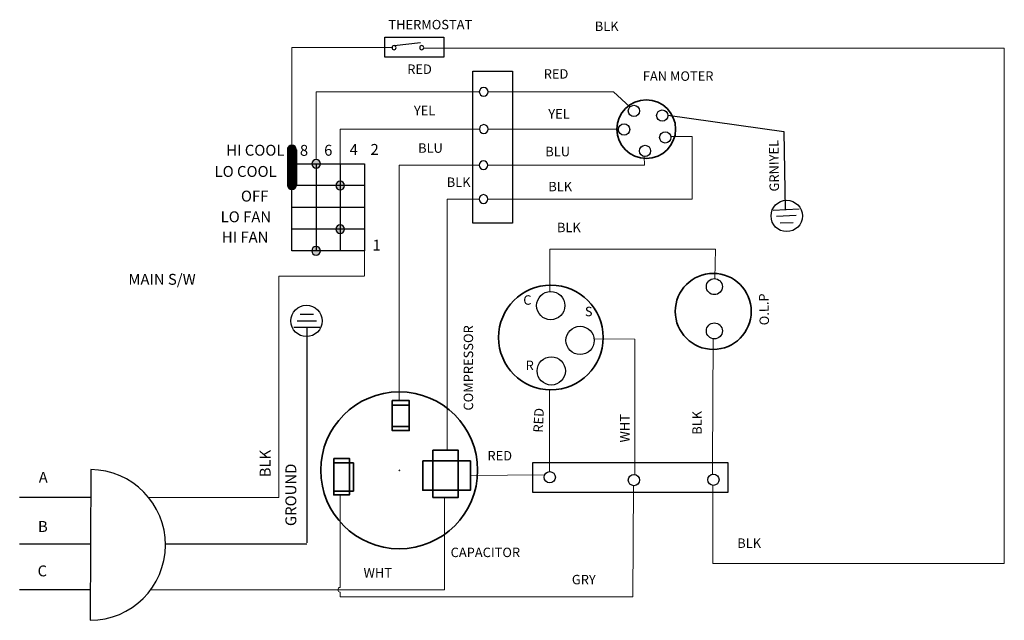
# Model space of a CAD drawing. Units: inches. Extents: x 2585 to 4283, y 904 to 1939.
import ezdxf

# ---------------------------------------------------------------- set-up
doc = ezdxf.new("R2010")
doc.units = ezdxf.units.IN
doc.header["$MEASUREMENT"] = 0
for name, color, linetype, lineweight in [('E-ANNO-TEXT', 7, 'Continuous', 25), ('E-POWR-EQPM', 7, 'Continuous', 35), ('E-POWR-GRND', 3, 'Continuous', 25), ('E-POWR-PATT', 7, 'Continuous', 13), ('E-POWR-SWCH', 7, 'Continuous', 30), ('E-POWR-TERM', 7, 'Continuous', 25), ('E-POWR-WIRE', 7, 'Continuous', 18), ('E-WIRE-TEXT', 7, 'Continuous', 18)]:
    doc.layers.add(name, color=color, linetype=linetype, lineweight=lineweight)
doc.styles.get("Standard").update_dxf_attribs({"font": 'arial.ttf'})

# ---------------------------------------------------------------- blocks, each defined once
blk = doc.blocks.new('Ground')
for p, q in [((-0.1, 0), (0.1, 0)), ((0.075, -0.05), (-0.075, -0.05)), ((-0.05, -0.1), (0.05, -0.1))]:
    blk.add_line(p, q)
blk = doc.blocks.new('GROUND-CIRCLED')
blk.add_circle((27, 27), 27)
at = {"xscale": 225.3922525633989, "yscale": 225.3922525633989, "zscale": 225.3922525633989, "rotation": 180}
blk.add_blockref('Ground', (27.6, 15.9), dxfattribs=at)
blk = doc.blocks.new('TERMINAL-STRIP-CONTACT')
blk.add_lwpolyline([(0, 7.5, 1), (15, 7.5, 1)], format="xyb", close=True)
blk = doc.blocks.new('TERMINAL-OPEN')
blk.add_circle((9.8, 9.8), 9.75)
blk = doc.blocks.new('SELECTOR-CONTACT')
blk.add_lwpolyline([(0, 7.5, 1), (15, 7.5, 1)], format="xyb", close=True)
blk = doc.blocks.new('COMPRESSOR-TERMINAL')
blk.add_circle((24.4, 24.4), 24.4)
blk = doc.blocks.new('OVERLOAD-TERMINAL')
blk.add_circle((13.8, 13.8), 13.8)

msp = doc.modelspace()

# ---------------------------------------------------------------- hatches: boundary and pattern name
at = {"layer": 'E-POWR-PATT'}
h = msp.add_hatch(dxfattribs=at)
h.set_pattern_fill('ANSI31', color=256)
h.set_pattern_definition([(45, (2034.52184, 1087.94078), (-0.088388348, 0.088388348), [])])
h.paths.add_polyline_path([(3054.4, 1690.8), (3054.4, 1722.8, 0.417432), (3046.6, 1715.1), (3046.6, 1654.3, 0.417432), (3054.4, 1646.6)])
h.paths.add_polyline_path([(3062.1, 1690.8), (3054.4, 1690.8), (3054.4, 1646.6, 0.411002), (3062.1, 1654.3)])
h.paths.add_polyline_path([(3062.1, 1715.1, 0.411002), (3054.4, 1722.8), (3054.4, 1690.8), (3062.1, 1690.8)])
h = msp.add_hatch(color=256, dxfattribs=at)
h.dxf.hatch_style = 1
h.paths.add_polyline_path([(3088.7, 1690.8), (3103.7, 1690.8, 1)])
h.paths.add_polyline_path([(3103.7, 1690.8), (3096.2, 1690.8), (3096.2, 1683.3, 0.414214)])
h.paths.add_polyline_path([(3096.2, 1690.8), (3088.7, 1690.8, 0.414214), (3096.2, 1683.3)])
h.paths.add_polyline_path([(3137.9, 1585.7, 0.414214), (3130.4, 1578.2), (3137.9, 1578.2)])
h.paths.add_polyline_path([(3137.9, 1585.7), (3137.9, 1578.2), (3145.4, 1578.2, 0.414214)])
h.paths.add_polyline_path([(3145.4, 1578.2), (3137.9, 1578.2), (3137.9, 1570.7, 0.414214)])
h.paths.add_polyline_path([(3137.9, 1578.2), (3130.4, 1578.2, 0.414214), (3137.9, 1570.7)])
h.paths.add_polyline_path([(3145.4, 1653.2), (3137.9, 1653.2), (3137.9, 1645.7, 0.414214)])
h.paths.add_polyline_path([(3137.9, 1653.2), (3130.4, 1653.2, 0.414214), (3137.9, 1645.7)])
h.paths.add_polyline_path([(3137.9, 1660.7, 0.414214), (3130.4, 1653.2), (3137.9, 1653.2)])
h.paths.add_polyline_path([(3137.9, 1660.7), (3137.9, 1653.2), (3145.4, 1653.2, 0.414214)])
h.paths.add_polyline_path([(3103.7, 1540.7), (3088.7, 1540.7, 1)])
h.paths.add_polyline_path([(3096.2, 1548.2), (3096.2, 1540.7), (3103.7, 1540.7, 0.414214)])
h.paths.add_polyline_path([(3096.2, 1548.2, 0.414214), (3088.7, 1540.7), (3096.2, 1540.7)])

# ---------------------------------------------------------------- linework, layer by layer
at = {"layer": 'E-POWR-EQPM'}
for p, q in [((3227.4, 1274.9), (3257.3, 1274.9)), ((3227.5, 1237.8), (3256.5, 1237.8)), ((3126.5, 1175), (3160.8, 1175)), ((3160.8, 1175), (3160.8, 1126.1)), ((3160.8, 1126.1), (3126.3, 1126.1))]:
    msp.add_line(p, q, dxfattribs=at)
for points in [[(3227.4, 1282.5), (3256.9, 1282.5), (3256.9, 1230.7), (3227.4, 1230.7)], [(3297.6, 1196.8), (3341.4, 1196.8), (3341.4, 1115.5), (3297.6, 1115.5)], [(3126.5, 1182.8), (3153.5, 1182.8), (3153.5, 1120), (3126.5, 1120)], [(3280.1, 1178.5), (3362.4, 1178.5), (3362.4, 1127.8), (3280.1, 1127.8)]]:
    msp.add_lwpolyline(points, close=True, dxfattribs=at)
for centre, radius in [((3665.7, 1750.4), 50.6), ((3781.2, 1436.3), 65.5), ((3501.1, 1391.3), 90.2), ((3239.5, 1162.3), 135.3), ((3239.8, 1162.3), 0.287)]:
    msp.add_circle(centre, radius, dxfattribs=at)
at = {"layer": 'E-POWR-GRND'}
for p, q in [((3702.9, 1774.4), (3902.7, 1746.4)), ((3902.7, 1746.5), (3905.3, 1611.8)), ((3080.4, 1408.5), (3080.4, 1340.3)), ((3080.4, 1344.6), (3080.4, 1037.1)), ((3080.4, 1034.9), (2836.3, 1034.9))]:
    msp.add_line(p, q, dxfattribs=at)
at = {"layer": 'E-POWR-SWCH'}
for p, q in [((3230.6, 1894.6), (3276.1, 1900.1)), ((3046.6, 1715.1), (3046.6, 1654.3)), ((3062.1, 1715.1), (3062.1, 1654.3)), ((3054.4, 1690.8), (3179.5, 1690.8)), ((3054.4, 1540.7), (3054.4, 1690.8)), ((3096.2, 1690.8), (3096.2, 1540.7)), ((3137.9, 1690.8), (3137.9, 1540.7)), ((3179.5, 1690.8), (3179.5, 1540.7)), ((3179.5, 1653.2), (3054.4, 1653.2)), ((3179.5, 1615.7), (3054.4, 1615.7)), ((3179.5, 1578.2), (3054.4, 1578.2)), ((3179.5, 1540.7), (3054.4, 1540.7))]:
    msp.add_line(p, q, dxfattribs=at)
msp.add_lwpolyline([(3214.9, 1908.9), (3316.3, 1908.9), (3316.3, 1874.6), (3214.9, 1874.6)], close=True, dxfattribs=at)
for points in [[(3227.1, 1891.1, 1), (3234.1, 1891.1, 1)], [(3274.9, 1891.1, 1), (3281.9, 1891.1, 1)]]:
    msp.add_lwpolyline(points, format="xyb", close=True, dxfattribs=at)
for centre, start, end in [((3054.3, 1715.1), 0, 180), ((3054.3, 1654.3), 180, 0)]:
    msp.add_arc(centre, 7.74, start, end, dxfattribs=at)
at = {"layer": 'E-POWR-TERM'}
for p, q in [((2707.6, 1163.5), (2706.4, 903.7)), ((2707.4, 1115.5), (2584.8, 1115.5)), ((2707, 1034.9), (2584.8, 1034.9)), ((2706.6, 956.3), (2584.8, 956.3))]:
    msp.add_line(p, q, dxfattribs=at)
for points in [[(3366.6, 1850.5), (3434.8, 1850.5), (3434.8, 1588.3), (3366.6, 1588.3)], [(3470, 1175.7), (3806.4, 1175.7), (3806.4, 1123.8), (3470, 1123.8)]]:
    msp.add_lwpolyline(points, close=True, dxfattribs=at)
msp.add_arc((2706.4, 1033.6), 129.9, 270, 89.4511, dxfattribs=at)
at = {"layer": 'E-POWR-WIRE'}
for p, q in [((3227.1, 1891.1), (3054.4, 1891.1)), ((3054.4, 1891.1), (3054.4, 1690.8)), ((3281.8, 1890.2), (4283.3, 1890.2)), ((4283.3, 1001.7), (4283.3, 1890.2)), ((3096.2, 1698.3), (3096.2, 1815)), ((3096.2, 1815), (3377.9, 1815)), ((3392.7, 1815), (3609.2, 1815)), ((3609.2, 1815), (3637.6, 1788.9)), ((3609.2, 1815), (3609.2, 1815)), ((3137.9, 1690.8), (3137.9, 1750.7)), ((3137.9, 1750.7), (3378.6, 1750.7)), ((3393.1, 1750.8), (3617.5, 1750.8)), ((3745, 1737.8), (3708, 1737.9)), ((3745, 1630.1), (3745, 1737.8)), ((3662.4, 1688.4), (3662.3, 1703.2)), ((3377.7, 1688.5), (3239.5, 1688.5)), ((3239.5, 1688.5), (3239.5, 1282.5)), ((3392.7, 1688.5), (3608.3, 1688.5)), ((3608.3, 1688.5), (3645.1, 1688.4)), ((3643.5, 1688.4), (3662.4, 1688.4)), ((3377.7, 1630.1), (3322.2, 1630.1)), ((3322.2, 1630.1), (3322.2, 1196.8)), ((3392.7, 1630.1), (3606.6, 1630.1)), ((3606.6, 1630.1), (3745, 1630.1)), ((3179.5, 1540.7), (3179.5, 1497.7)), ((3499.2, 1543.4), (3499.1, 1470.6)), ((3779.9, 1543.4), (3499.2, 1543.4)), ((3779.3, 1543.4), (3784.9, 1543.4)), ((3784.9, 1543.4), (3783.9, 1492.8)), ((3179.5, 1497.2), (3032.1, 1497.2)), ((3032.1, 1497.2), (3032.1, 1115.5)), ((3646, 1388.4), (3575.8, 1389.1)), ((3646, 1155), (3646, 1388.4)), ((3779.9, 1175.5), (3780.8, 1389)), ((3498.8, 1301.1), (3498.8, 1159.9)), ((3779.9, 1155.6), (3779.9, 1175.7)), ((3362.4, 1153.6), (3490.2, 1154.3)), ((3642.4, 944.1), (3643.8, 1135.7)), ((3780.7, 1136.3), (3780.7, 1001.7)), ((3032.1, 1115.5), (2807.2, 1115.5)), ((3137.6, 1120), (3137.6, 960.3)), ((3317.7, 1115.5), (3317.7, 956.3)), ((3780.7, 1001.7), (4283.3, 1001.7)), ((3317.7, 956.3), (2810.8, 956.3)), ((3137.6, 952.2), (3137.6, 944.1)), ((3137.6, 944.1), (3642.4, 944.1))]:
    msp.add_line(p, q, dxfattribs=at)
msp.add_arc((3137.7, 956.3), 4.04, 91.3808, 268.6192, dxfattribs=at)

# ---------------------------------------------------------------- block references
at = {"layer": 'E-POWR-GRND', "rotation": 182.5618974607787}
msp.add_blockref('GROUND-CIRCLED', (3933.7, 1629), dxfattribs=at)
at = {"layer": 'E-POWR-GRND'}
msp.add_blockref('GROUND-CIRCLED', (3052.5, 1392.8), dxfattribs=at)
at = {"layer": 'E-POWR-SWCH'}
msp.add_blockref('SELECTOR-CONTACT', (3088.7, 1683.3), dxfattribs=at)
at = {"layer": 'E-POWR-SWCH', "rotation": 180}
for p in [(3145.1, 1660.7), (3145.1, 1585.7), (3103.5, 1548.2)]:
    msp.add_blockref('SELECTOR-CONTACT', p, dxfattribs=at)
at = {"layer": 'E-POWR-TERM'}
for name, p in [('TERMINAL-STRIP-CONTACT', (3377.7, 1807.5)), ('TERMINAL-OPEN', (3634.6, 1772.1)), ('TERMINAL-OPEN', (3683.4, 1764.1)), ('TERMINAL-OPEN', (3617.5, 1740.1)), ('TERMINAL-OPEN', (3688.6, 1726.5)), ('TERMINAL-OPEN', (3653.7, 1703.2)), ('OVERLOAD-TERMINAL', (3769.3, 1465.2)), ('COMPRESSOR-TERMINAL', (3476.5, 1421.9)), ('COMPRESSOR-TERMINAL', (3527.2, 1361.8)), ('OVERLOAD-TERMINAL', (3769.3, 1388.8)), ('COMPRESSOR-TERMINAL', (3477.4, 1309.3)), ('TERMINAL-OPEN', (3489.3, 1140.4)), ('TERMINAL-OPEN', (3634.6, 1135.6)), ('TERMINAL-OPEN', (3771.7, 1136.2))]:
    msp.add_blockref(name, p, dxfattribs=at)
at = {"layer": 'E-POWR-TERM', "rotation": 180}
for p in [(3392.8, 1758.3), (3392.5, 1696), (3392.5, 1637.6)]:
    msp.add_blockref('TERMINAL-STRIP-CONTACT', p, dxfattribs=at)

# ---------------------------------------------------------------- texts
at = {"layer": 'E-ANNO-TEXT'}
for s, height, p in [('THERMOSTAT', 16.29, (3220.9, 1922.7)), ('FAN MOTER', 16.29, (3659.7, 1833.9)), ('HI COOL', 18.81, (2941.2, 1704.8)), ('8', 18.8, (3068.2, 1704.6)), ('6', 18.8, (3110, 1704.8)), ('4', 18.8, (3154, 1705.9)), ('2', 18.8, (3190, 1706.2)), ('LO COOL', 18.81, (2921, 1668.2)), ('OFF', 18.81, (2966.5, 1625.7)), ('LO FAN', 18.81, (2931.5, 1590)), ('HI FAN', 18.81, (2933.6, 1555)), ('1', 18.8, (3193.4, 1541.1)), ('MAIN S/W', 18.81, (2772.3, 1482.2)), ('C', 16.3, (3453.5, 1447.8)), ('S', 16.3, (3559.7, 1428)), ('R', 16.3, (3457.6, 1335)), ('A', 18.8, (2617.7, 1140.7)), ('B', 18.8, (2616.4, 1056)), ('CAPACITOR', 16.29, (3328.2, 1012.6)), ('C', 18.8, (2615.7, 979.4))]:
    msp.add_text(s, height=height, dxfattribs=at).set_placement(p)
for s, rotation, p in [('O.L.P', 91.2279, (3877.5, 1412.5)), ('COMPRESSOR', 90, (3367, 1265.3))]:
    msp.add_text(s, height=16.29, rotation=rotation, dxfattribs=at).set_placement(p)
at = {"layer": 'E-WIRE-TEXT'}
for s, p in [('BLK', (3576.8, 1919.8)), ('RED', (3253.3, 1845.8)), ('RED', (3488.8, 1837.7)), ('YEL', (3264.8, 1774.6)), ('YEL', (3496.7, 1768.8)), ('BLU', (3272.1, 1709.8)), ('BLU', (3491.5, 1703.8)), ('BLK', (3321.5, 1650.9)), ('BLK', (3496.7, 1643.4)), ('BLK', (3511.7, 1572.9)), ('RED', (3391.7, 1179.3)), ('BLK', (3822.6, 1028.5)), ('WHT', (3178, 977.4)), ('GRY', (3537.3, 965.7))]:
    msp.add_text(s, height=16.29, dxfattribs=at).set_placement(p)
for s, height, rotation, p in [('GRNIYEL', 16.29, 90.6442, (3894.7, 1643.1)), ('RED', 16.29, 87.1355, (3487, 1226.9)), ('WHT', 16.29, 90, (3636.8, 1210.3)), ('BLK', 16.29, 90, (3761.4, 1223.6)), ('BLK', 18.81, 90, (3017.7, 1150.3)), ('GROUND', 18.81, 90, (3062, 1066.1))]:
    msp.add_text(s, height=height, rotation=rotation, dxfattribs=at).set_placement(p)

doc.saveas('drawing.dxf')
